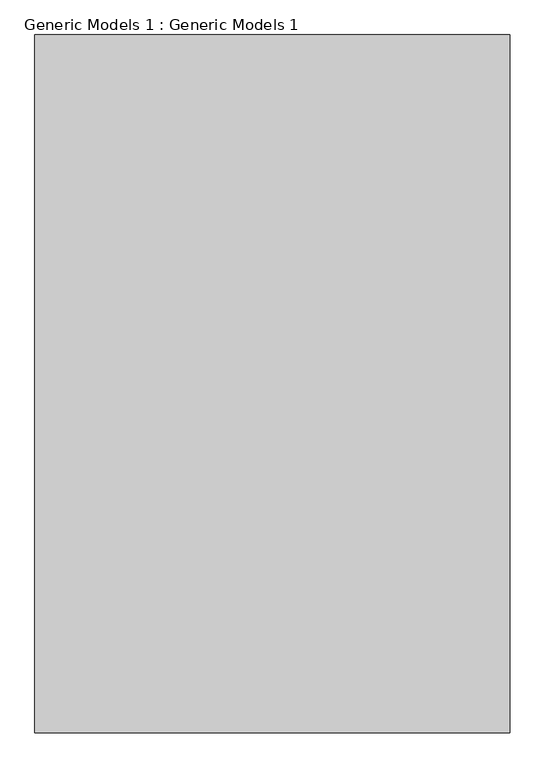
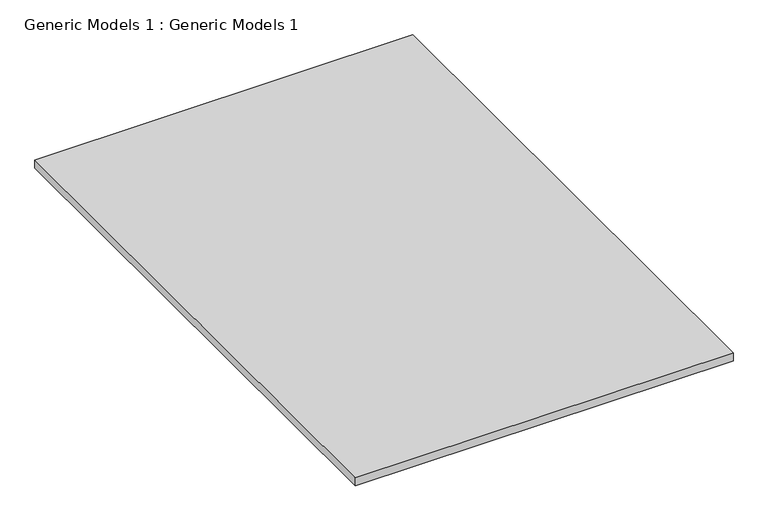
"""IFC4 building model written with IfcOpenShell, lengths in millimetres: proxy geometry, Generic Models 1 : Generic Models 1."""

from ifc_helpers import new_model, si_unit, frame, origin, place, context, project, spatial, polyline, outline, extrude, source, transform, mapped, element, save


def generic_models_1_generic_models_1_f513481b(model_context):
    return source(origin(), model_context, "Body", "SweptSolid", [
        extrude(outline(polyline([(-4407.329521, 3660.3958868), (-4407.329521, -16169.6001929), (-17905.1468092, -16169.6001929), (-17905.1468092, 3660.3958868), (-4407.329521, 3660.3958868)])), frame((0.0, 0.0, -304.8), z_axis=(0.0, 0.0, 1.0), x_axis=(1.0, 0.0, 0.0)), (0.0, 0.0, 1.0), 304.8),
    ])


if __name__ == "__main__":
    model = new_model("IFC4")
    model_context = context("Model", 3, world=origin())
    ifc_project = project(units=[si_unit("LENGTHUNIT", "METRE", prefix="MILLI")], contexts=[model_context])
    site = spatial("IfcSite", under=ifc_project)
    building = spatial("IfcBuilding", under=site)
    placement = place(None, origin())
    generic_models_1_generic_models_1_shape = generic_models_1_generic_models_1_f513481b(model_context)
    element("IfcBuildingElementProxy", 1, Name="Generic Models 1 : Generic Models 1", ObjectType="Generic Models 1 : Generic Models 1", at=placement, inside=building, context=model_context, shape_type="MappedRepresentation", body=[
        mapped(generic_models_1_generic_models_1_shape, transform((0.0, 0.0, 0.0), x_axis=(1.0, 0.0, 0.0), y_axis=(0.0, 1.0, 0.0), z_axis=(0.0, 0.0, 1.0))),
    ])
    save(model, "model.ifc")
